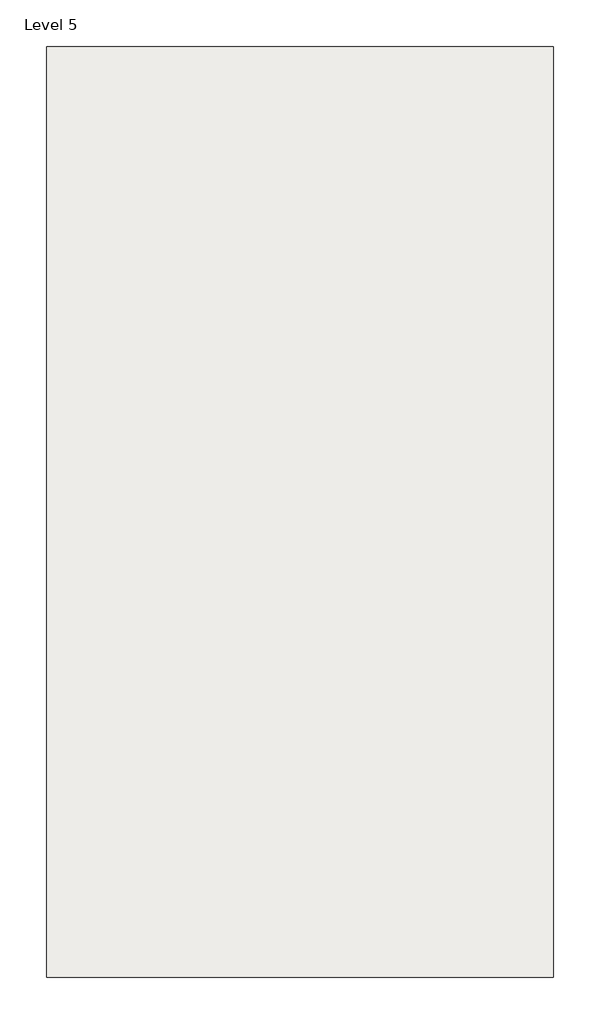
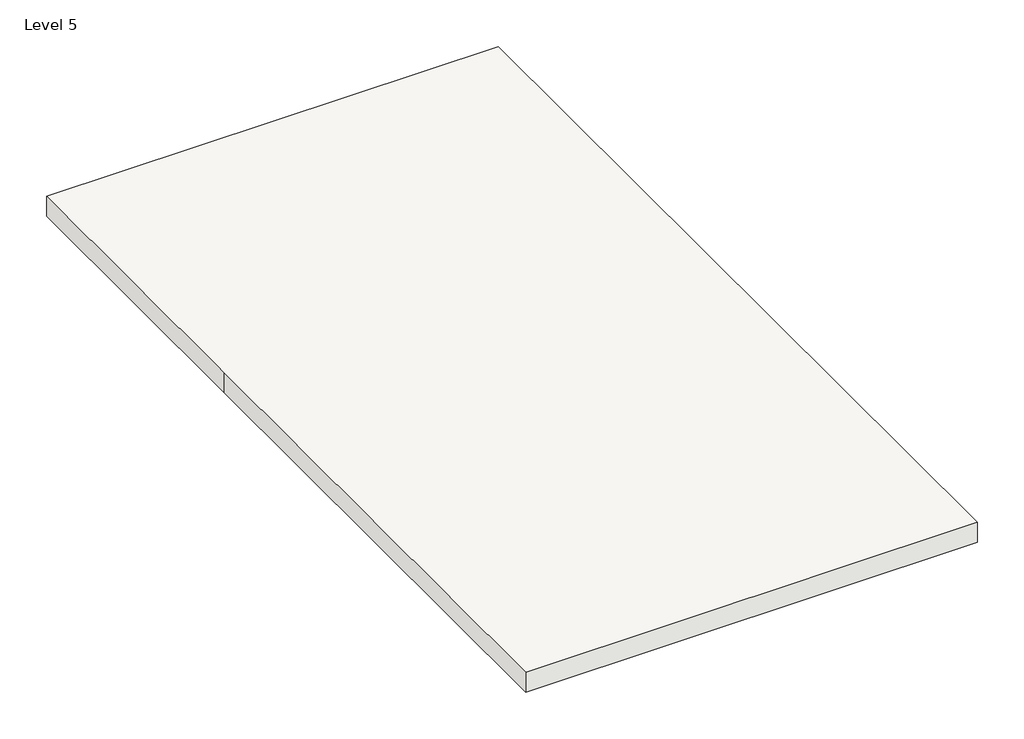
# One storey: 1 roof.
"""IFC4 building model written with IfcOpenShell, lengths in millimetres."""

from ifc_helpers import new_model, si_unit, frame, origin, place, context, project, spatial, polyline, outline, extrude, element, save

model = new_model("IFC4")

# Units and contexts
model_context = context("Model", 3, world=origin())
ifc_project = project(units=[si_unit("LENGTHUNIT", "METRE", prefix="MILLI")], contexts=[model_context])

# Site, building, storey
site = spatial("IfcSite", under=ifc_project)
building = spatial("IfcBuilding", under=site)
storey = spatial("IfcBuildingStorey", under=building, Name="Level 5", Elevation=14630.4)

# Roof
placement = place(None, origin())
element("IfcRoof", 1, ObjectType="Generic - 12\"", at=placement, inside=storey, context=model_context, shape_type="SweptSolid", body=[
    extrude(outline(polyline([(-5043.2745124, 11142.1609482), (1452.7754876, 11142.1609482), (1452.7754876, -783.1390518), (-5043.2745124, -783.1390518), (-5043.2745124, 6735.2609482), (-5043.2745124, 11142.1609482)])), frame((0.0, 0.0, 14630.4), z_axis=(0.0, 0.0, 1.0), x_axis=(1.0, 0.0, 0.0)), (0.0, 0.0, 1.0), 304.8),
])

save(model, "model.ifc")

# Revit data of these elements
# Type "Generic - 12\""
#   Assembly Code = "B1020"
#   Layers, outside or top first: 1' - 0" no material (function 1)
# Element 1 (IfcRoof, "Generic - 12\"")
#   built-in parameter 1001705 = 49 (stored number, unit not read)
#   built-in parameter 1001710 = 33615
#   Phase Created = New Construction
#   Materials on its faces: "Default Roof"
# Materials
#   "Default Roof": colour RGB 88 101 114, transparency 0
